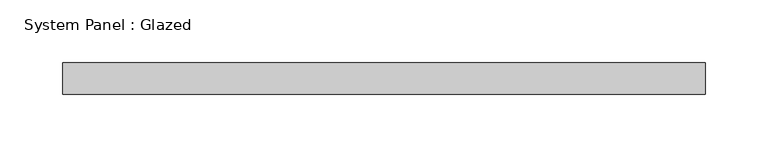
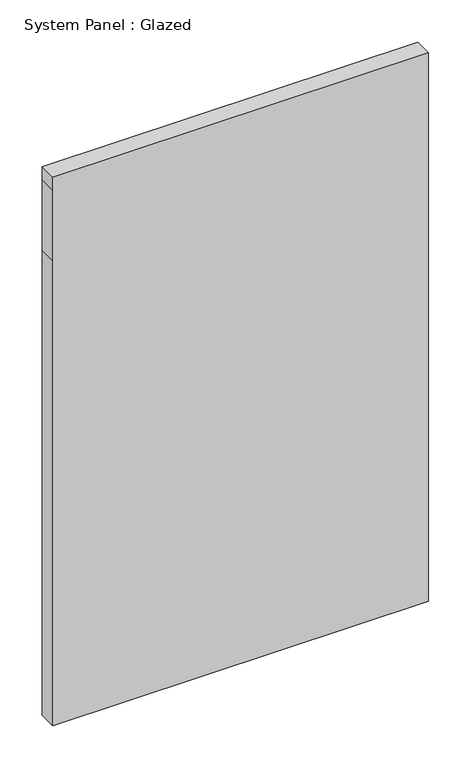
"""IFC4 building model written with IfcOpenShell, lengths in millimetres: plate geometry, System Panel : Glazed."""

from ifc_helpers import new_model, si_unit, frame, origin, place, context, project, spatial, polyline, outline, extrude, source, transform, mapped, element, save


def system_panel_glazed_2d09ef22(model_context):
    return source(origin(), model_context, "Body", "SweptSolid", [
        extrude(outline(polyline([(0.0, -257.175), (0.0, 257.175), (672.7967564, 257.175), (774.3967564, 257.175), (793.4467564, 257.175), (793.4467564, -257.175), (774.3967564, -257.175), (672.7967564, -257.175), (0.0, -257.175)])), frame((0.0, 19.05, 0.0), z_axis=(0.0, 1.0, 0.0), x_axis=(0.0, 0.0, 1.0)), (0.0, 0.0, 1.0), 25.4),
    ])


if __name__ == "__main__":
    model = new_model("IFC4")
    model_context = context("Model", 3, world=origin())
    ifc_project = project(units=[si_unit("LENGTHUNIT", "METRE", prefix="MILLI")], contexts=[model_context])
    site = spatial("IfcSite", under=ifc_project)
    building = spatial("IfcBuilding", under=site)
    placement = place(None, origin())
    system_panel_glazed_shape = system_panel_glazed_2d09ef22(model_context)
    element("IfcPlate", 1, ObjectType="System Panel : Glazed", at=placement, inside=building, context=model_context, shape_type="MappedRepresentation", body=[
        mapped(system_panel_glazed_shape, transform((0.0, 0.0, 0.0), x_axis=(1.0, 0.0, 0.0), y_axis=(0.0, 1.0, 0.0), z_axis=(0.0, 0.0, 1.0))),
    ])
    save(model, "model.ifc")

# Revit data of these elements
# Type "System Panel : Glazed"
#   Construction Type Id = "GSP4R"
#   Analytic Construction = "1/8 in Pilkington single glazing"
#   Visual Light Transmittance = 0.9
#   Solar Heat Gain Coefficient = 0.86
#   Heat Transfer Coefficient (U) = 1.18115 BTU/(h·ft²·°F)
#   Define Thermal Properties by = 1
# Element 1 (IfcPlate, "System Panel : Glazed")
#   Materials on its faces: "Glass"
# Materials
#   "Glass": class "Glass", colour RGB 0 128 192, transparency 0.75, Description = "Soda Lime Glass", Cost = 0
